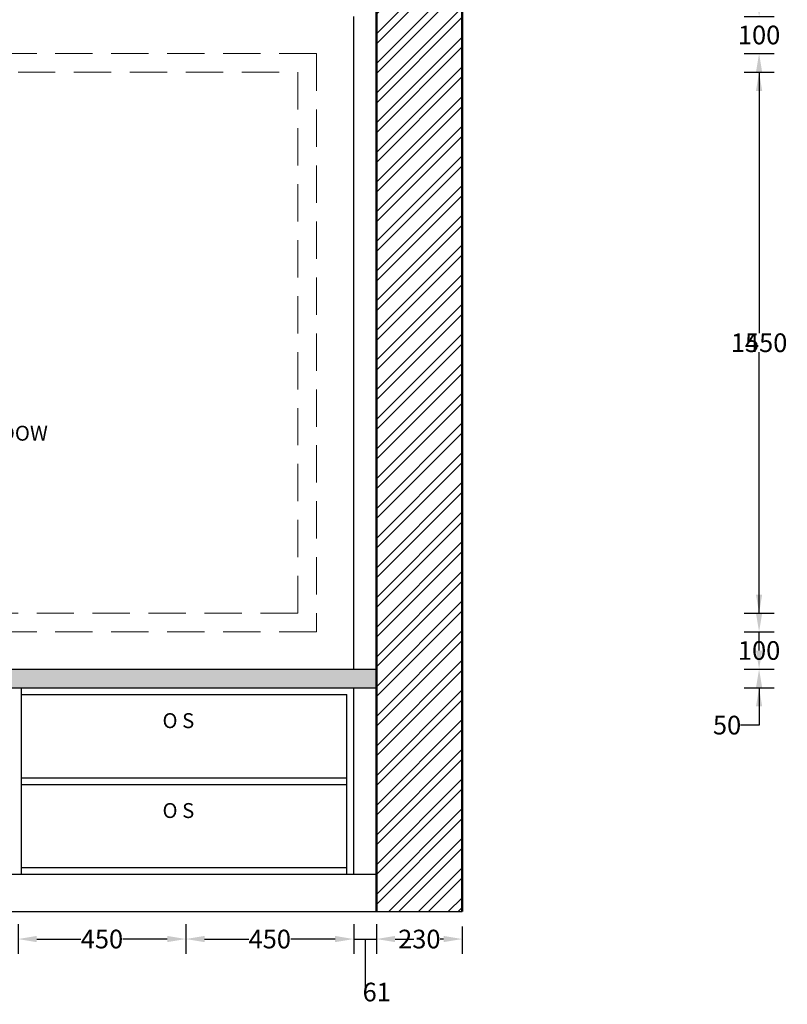
# Model space of a CAD drawing. Units: millimetres. Extents: x -472 to 16192, y -4730 to 4331.
# Tile 7 of 8: x 14134 to 16192, y -4534 to -1895. Entities that reach past the tile are written whole.
import ezdxf

# ---------------------------------------------------------------- set-up
doc = ezdxf.new("R2010")
doc.units = ezdxf.units.MM
doc.header["$MEASUREMENT"] = 0
doc.linetypes.add('DASHED', pattern=[0.75, 0.5, -0.25])
for name, color, linetype, lineweight in [('A-ANNO-DIMS', 2, 'Continuous', 18), ('A-ANNO-TEXT', 6, 'Continuous', 18), ('A-ELEV', 7, 'Continuous', 25), ('A-GLAZ', 4, 'DASHED', 18), ('A-WALL', 7, 'Continuous', 50), ('A-WALL-PATT', 8, 'Continuous', 13)]:
    doc.layers.add(name, color=color, linetype=linetype, lineweight=lineweight)
doc.styles.get("Standard").update_dxf_attribs({"font": 'arial.ttf'})
doc.dimstyles.get("Standard").update_dxf_attribs({"dimtxt": 50, "dimasz": 50, "dimexe": 40, "dimexo": 40, "dimgap": 0.09, "dimtad": 0, "dimtih": 1, "dimtoh": 1, "dimdec": 0, "dimzin": 0, "dimdsep": 46, "dimtxsty": 'Standard', "dimcen": 0.09, "dimclrd": 1, "dimclre": 3, "dimclrt": 6, "dimadec": 0, "dimazin": 0, "dimtfac": 1, "dimtdec": 0, "dimtofl": 0, "dimtmove": 0, "dimatfit": 3, "dimfxl": 40, "dimfxlon": 1, "dimtolj": 1, "dimtzin": 0, "dimarcsym": 0})

# ---------------------------------------------------------------- blocks, each defined once
blk = doc.blocks.new('*D61')
at = {"layer": 'A-ANNO-DIMS', "color": 0, "lineweight": -2, "transparency": 16777216}
for p, q in [((14129.7, -4319.4), (14129.7, -4399.4)), ((14579.7, -4319.4), (14579.7, -4399.4)), ((14179.7, -4359.4), (14298.4, -4359.4)), ((14529.7, -4359.4), (14410.9, -4359.4))]:
    blk.add_line(p, q, dxfattribs=at)
at = {"layer": 'A-ANNO-DIMS', "color": 0, "transparency": 16777216}
for points in [[(14179.7, -4351), (14179.7, -4367.7), (14129.7, -4359.4)], [(14529.7, -4351), (14529.7, -4367.7), (14579.7, -4359.4)]]:
    blk.add_solid(points, dxfattribs=at)
at = {"layer": 'Defpoints', "color": 0, "transparency": 16777216}
for p in [(14129.7, -4185.9), (14579.7, -4185.9), (14579.7, -4359.4)]:
    blk.add_point(p, dxfattribs=at)
at = {"layer": 'A-ANNO-DIMS', "color": 0, "transparency": 16777216, "insert": (14354.7, -4359.4), "char_height": 50, "attachment_point": 5}
blk.add_mtext('\\A1;450', dxfattribs=at)
blk = doc.blocks.new('*D62')
at = {"layer": 'A-ANNO-DIMS', "color": 0, "lineweight": -2, "transparency": 16777216}
for p, q in [((14579.7, -4319.4), (14579.7, -4399.4)), ((15029.7, -4319.4), (15029.7, -4399.4)), ((14629.7, -4359.4), (14748.4, -4359.4)), ((14979.7, -4359.4), (14860.9, -4359.4))]:
    blk.add_line(p, q, dxfattribs=at)
at = {"layer": 'A-ANNO-DIMS', "color": 0, "transparency": 16777216}
for points in [[(14629.7, -4351), (14629.7, -4367.7), (14579.7, -4359.4)], [(14979.7, -4351), (14979.7, -4367.7), (15029.7, -4359.4)]]:
    blk.add_solid(points, dxfattribs=at)
at = {"layer": 'Defpoints', "color": 0, "transparency": 16777216}
for p in [(14579.7, -4185.9), (15029.7, -4185.9), (15029.7, -4359.4)]:
    blk.add_point(p, dxfattribs=at)
at = {"layer": 'A-ANNO-DIMS', "color": 0, "transparency": 16777216, "insert": (14804.7, -4359.4), "char_height": 50, "attachment_point": 5}
blk.add_mtext('\\A1;450', dxfattribs=at)
blk = doc.blocks.new('*D63')
at = {"layer": 'A-ANNO-DIMS', "color": 0, "lineweight": -2, "transparency": 16777216}
for p, q in [((15029.7, -4319.4), (15029.7, -4399.4)), ((15090.7, -4319.4), (15090.7, -4399.4)), ((14979.7, -4359.4), (14929.7, -4359.4)), ((15029.7, -4359.4), (15090.7, -4359.4)), ((15060.2, -4359.4), (15060.2, -4501.5)), ((15140.7, -4359.4), (15190.7, -4359.4)), ((15060.2, -4501.5), (15060.3, -4501.5))]:
    blk.add_line(p, q, dxfattribs=at)
at = {"layer": 'A-ANNO-DIMS', "color": 0, "transparency": 16777216}
for points in [[(14979.7, -4351), (14979.7, -4367.7), (15029.7, -4359.4)], [(15140.7, -4351), (15140.7, -4367.7), (15090.7, -4359.4)]]:
    blk.add_solid(points, dxfattribs=at)
at = {"layer": 'Defpoints', "color": 0, "transparency": 16777216}
for p in [(15029.7, -4185.9), (15090.7, -4185.9), (15090.7, -4359.4)]:
    blk.add_point(p, dxfattribs=at)
at = {"layer": 'A-ANNO-DIMS', "color": 0, "transparency": 16777216, "insert": (15091.5, -4501.5), "char_height": 50, "attachment_point": 5}
blk.add_mtext('\\A1;61', dxfattribs=at)
blk = doc.blocks.new('*D64')
at = {"layer": 'A-ANNO-DIMS', "color": 0, "lineweight": -2, "transparency": 16777216}
for p, q in [((15090.7, -4319.4), (15090.7, -4399.4)), ((15320.7, -4325.9), (15320.7, -4399.4)), ((15140.7, -4359.4), (15150, -4359.4)), ((15270.7, -4359.4), (15261.3, -4359.4))]:
    blk.add_line(p, q, dxfattribs=at)
at = {"layer": 'A-ANNO-DIMS', "color": 0, "transparency": 16777216}
for points in [[(15140.7, -4351), (15140.7, -4367.7), (15090.7, -4359.4)], [(15270.7, -4351), (15270.7, -4367.7), (15320.7, -4359.4)]]:
    blk.add_solid(points, dxfattribs=at)
at = {"layer": 'Defpoints', "color": 0, "transparency": 16777216}
for p in [(15090.7, -4185.9), (15320.7, -4285.9), (15320.7, -4359.4)]:
    blk.add_point(p, dxfattribs=at)
at = {"layer": 'A-ANNO-DIMS', "color": 0, "transparency": 16777216, "insert": (15205.7, -4359.4), "char_height": 50, "attachment_point": 5}
blk.add_mtext('\\A1;230', dxfattribs=at)
blk = doc.blocks.new('*D100')
at = {"layer": 'A-ANNO-DIMS', "color": 1, "lineweight": -2, "transparency": 16777216}
for p, q in [((16116.7, -1835.9), (16116.7, -1785.9)), ((16116.7, -2035.9), (16116.7, -2085.9))]:
    blk.add_line(p, q, dxfattribs=at)
at = {"layer": 'A-ANNO-DIMS', "color": 3, "lineweight": -2, "transparency": 16777216}
for p, q in [((16076.7, -1885.9), (16156.7, -1885.9)), ((16076.7, -1985.9), (16156.7, -1985.9))]:
    blk.add_line(p, q, dxfattribs=at)
at = {"layer": 'A-ANNO-DIMS', "color": 1, "transparency": 16777216}
for points in [[(16108.3, -1835.9), (16125, -1835.9), (16116.7, -1885.9)], [(16108.3, -2035.9), (16125, -2035.9), (16116.7, -1985.9)]]:
    blk.add_solid(points, dxfattribs=at)
at = {"layer": 'Defpoints', "color": 0, "transparency": 16777216}
for p in [(5309, -1885.9), (5209, -1985.9), (16116.7, -1985.9)]:
    blk.add_point(p, dxfattribs=at)
at = {"layer": 'A-ANNO-DIMS', "color": 6, "transparency": 16777216, "insert": (16116.7, -1935.9), "char_height": 50, "attachment_point": 5}
blk.add_mtext('\\A1;100', dxfattribs=at)
blk = doc.blocks.new('*D101')
at = {"layer": 'A-ANNO-DIMS', "color": 3, "lineweight": -2, "transparency": 16777216}
for p, q in [((16076.7, -1985.9), (16156.7, -1985.9)), ((16076.7, -3535.9), (16156.7, -3535.9))]:
    blk.add_line(p, q, dxfattribs=at)
at = {"layer": 'A-ANNO-DIMS', "color": 1, "lineweight": -2, "transparency": 16777216}
for p, q in [((16116.7, -2035.9), (16116.7, -2735.3)), ((16116.7, -3485.9), (16116.7, -2786.5))]:
    blk.add_line(p, q, dxfattribs=at)
at = {"layer": 'A-ANNO-DIMS', "color": 1, "transparency": 16777216}
for points in [[(16108.3, -2035.9), (16125, -2035.9), (16116.7, -1985.9)], [(16108.3, -3485.9), (16125, -3485.9), (16116.7, -3535.9)]]:
    blk.add_solid(points, dxfattribs=at)
at = {"layer": 'Defpoints', "color": 0, "transparency": 16777216}
for p in [(5209, -1985.9), (5209, -3535.9), (16116.7, -3535.9)]:
    blk.add_point(p, dxfattribs=at)
at = {"layer": 'A-ANNO-DIMS', "color": 6, "transparency": 16777216, "insert": (16116.7, -2760.9), "char_height": 50, "attachment_point": 5}
blk.add_mtext('\\A1;1550', dxfattribs=at)
blk = doc.blocks.new('*D102')
at = {"layer": 'A-ANNO-DIMS', "color": 3, "lineweight": -2, "transparency": 16777216}
for p, q in [((16076.7, -2035.9), (16156.7, -2035.9)), ((16076.7, -3485.9), (16156.7, -3485.9))]:
    blk.add_line(p, q, dxfattribs=at)
at = {"layer": 'A-ANNO-DIMS', "color": 1, "lineweight": -2, "transparency": 16777216}
for p, q in [((16116.7, -2085.9), (16116.7, -2735.3)), ((16116.7, -3435.9), (16116.7, -2786.5))]:
    blk.add_line(p, q, dxfattribs=at)
at = {"layer": 'A-ANNO-DIMS', "color": 1, "transparency": 16777216}
for points in [[(16108.3, -2085.9), (16125, -2085.9), (16116.7, -2035.9)], [(16108.3, -3435.9), (16125, -3435.9), (16116.7, -3485.9)]]:
    blk.add_solid(points, dxfattribs=at)
at = {"layer": 'Defpoints', "color": 0, "transparency": 16777216}
for p in [(5159, -2035.9), (5159, -3485.9), (16116.7, -3485.9)]:
    blk.add_point(p, dxfattribs=at)
at = {"layer": 'A-ANNO-DIMS', "color": 6, "transparency": 16777216, "insert": (16116.7, -2760.9), "char_height": 50, "attachment_point": 5}
blk.add_mtext('\\A1;1450', dxfattribs=at)
blk = doc.blocks.new('*D103')
at = {"layer": 'A-ANNO-DIMS', "color": 1, "lineweight": -2, "transparency": 16777216}
for p, q in [((16116.7, -3485.9), (16116.7, -3435.9)), ((16116.7, -3685.9), (16116.7, -3735.9))]:
    blk.add_line(p, q, dxfattribs=at)
at = {"layer": 'A-ANNO-DIMS', "color": 3, "lineweight": -2, "transparency": 16777216}
for p, q in [((16076.7, -3535.9), (16156.7, -3535.9)), ((16076.7, -3635.9), (16156.7, -3635.9))]:
    blk.add_line(p, q, dxfattribs=at)
at = {"layer": 'A-ANNO-DIMS', "color": 1, "transparency": 16777216}
for points in [[(16108.3, -3485.9), (16125, -3485.9), (16116.7, -3535.9)], [(16108.3, -3685.9), (16125, -3685.9), (16116.7, -3635.9)]]:
    blk.add_solid(points, dxfattribs=at)
at = {"layer": 'Defpoints', "color": 0, "transparency": 16777216}
for p in [(5209, -3535.9), (5309, -3635.9), (16116.7, -3635.9)]:
    blk.add_point(p, dxfattribs=at)
at = {"layer": 'A-ANNO-DIMS', "color": 6, "transparency": 16777216, "insert": (16116.7, -3585.9), "char_height": 50, "attachment_point": 5}
blk.add_mtext('\\A1;100', dxfattribs=at)
blk = doc.blocks.new('*D104')
at = {"layer": 'A-ANNO-DIMS', "color": 1, "lineweight": -2, "transparency": 16777216}
for p, q in [((16116.7, -3585.9), (16116.7, -3535.9)), ((16116.7, -3735.9), (16116.7, -3785.9)), ((16116.7, -3785.9), (16066.7, -3785.9))]:
    blk.add_line(p, q, dxfattribs=at)
at = {"layer": 'A-ANNO-DIMS', "color": 3, "lineweight": -2, "transparency": 16777216}
for p, q in [((16076.7, -3635.9), (16156.7, -3635.9)), ((16076.7, -3685.9), (16156.7, -3685.9))]:
    blk.add_line(p, q, dxfattribs=at)
at = {"layer": 'A-ANNO-DIMS', "color": 1, "transparency": 16777216}
for points in [[(16108.3, -3585.9), (16125, -3585.9), (16116.7, -3635.9)], [(16108.3, -3735.9), (16125, -3735.9), (16116.7, -3685.9)]]:
    blk.add_solid(points, dxfattribs=at)
at = {"layer": 'Defpoints', "color": 0, "transparency": 16777216}
for p in [(5309, -3635.9), (5309, -3685.9), (16116.7, -3685.9)]:
    blk.add_point(p, dxfattribs=at)
at = {"layer": 'A-ANNO-DIMS', "color": 6, "transparency": 16777216, "insert": (16030.8, -3785.9), "char_height": 50, "attachment_point": 5}
blk.add_mtext('\\A1;50', dxfattribs=at)
blk = doc.blocks.new('*D105')
at = {"layer": 'A-ANNO-DIMS', "color": 3, "lineweight": -2, "transparency": 16777216}
for p, q in [((14929.7, -534.9), (14929.7, -454.9)), ((15029.7, -534.9), (15029.7, -454.9))]:
    blk.add_line(p, q, dxfattribs=at)
at = {"layer": 'A-ANNO-DIMS', "color": 1, "lineweight": -2, "transparency": 16777216}
for p, q in [((14879.7, -494.9), (14829.7, -494.9)), ((15079.7, -494.9), (15129.7, -494.9))]:
    blk.add_line(p, q, dxfattribs=at)
at = {"layer": 'A-ANNO-DIMS', "color": 1, "transparency": 16777216}
for points in [[(14879.7, -486.6), (14879.7, -503.2), (14929.7, -494.9)], [(15079.7, -486.6), (15079.7, -503.2), (15029.7, -494.9)]]:
    blk.add_solid(points, dxfattribs=at)
at = {"layer": 'Defpoints', "color": 0, "transparency": 16777216}
for p in [(15029.7, -494.9), (15029.7, -1885.9), (14929.7, -1985.9)]:
    blk.add_point(p, dxfattribs=at)
at = {"layer": 'A-ANNO-DIMS', "color": 6, "transparency": 16777216, "insert": (15182.5, -494.9), "char_height": 50, "attachment_point": 5}
blk.add_mtext('\\A1;100', dxfattribs=at)
blk = doc.blocks.new('*D106')
at = {"layer": 'A-ANNO-DIMS', "color": 3, "lineweight": -2, "transparency": 16777216}
for p, q in [((13329.7, -534.9), (13329.7, -454.9)), ((14929.7, -534.9), (14929.7, -454.9))]:
    blk.add_line(p, q, dxfattribs=at)
at = {"layer": 'A-ANNO-DIMS', "color": 1, "lineweight": -2, "transparency": 16777216}
for p, q in [((13379.7, -494.9), (14057.3, -494.9)), ((14879.7, -494.9), (14202, -494.9))]:
    blk.add_line(p, q, dxfattribs=at)
at = {"layer": 'A-ANNO-DIMS', "color": 1, "transparency": 16777216}
for points in [[(13379.7, -486.6), (13379.7, -503.2), (13329.7, -494.9)], [(14879.7, -486.6), (14879.7, -503.2), (14929.7, -494.9)]]:
    blk.add_solid(points, dxfattribs=at)
at = {"layer": 'Defpoints', "color": 0, "transparency": 16777216}
for p in [(14929.7, -494.9), (13329.7, -1985.9), (14929.7, -1985.9)]:
    blk.add_point(p, dxfattribs=at)
at = {"layer": 'A-ANNO-DIMS', "color": 6, "transparency": 16777216, "insert": (14129.7, -494.9), "char_height": 50, "attachment_point": 5}
blk.add_mtext('\\A1;1600', dxfattribs=at)
blk = doc.blocks.new('*D107')
at = {"layer": 'A-ANNO-DIMS', "color": 3, "lineweight": -2, "transparency": 16777216}
for p, q in [((13379.7, -534.9), (13379.7, -454.9)), ((14879.7, -534.9), (14879.7, -454.9))]:
    blk.add_line(p, q, dxfattribs=at)
at = {"layer": 'A-ANNO-DIMS', "color": 1, "lineweight": -2, "transparency": 16777216}
for p, q in [((13429.7, -494.9), (14057.3, -494.9)), ((14829.7, -494.9), (14202, -494.9))]:
    blk.add_line(p, q, dxfattribs=at)
at = {"layer": 'A-ANNO-DIMS', "color": 1, "transparency": 16777216}
for points in [[(13429.7, -486.6), (13429.7, -503.2), (13379.7, -494.9)], [(14829.7, -486.6), (14829.7, -503.2), (14879.7, -494.9)]]:
    blk.add_solid(points, dxfattribs=at)
at = {"layer": 'Defpoints', "color": 0, "transparency": 16777216}
for p in [(14879.7, -494.9), (13379.7, -2035.9), (14879.7, -2035.9)]:
    blk.add_point(p, dxfattribs=at)
at = {"layer": 'A-ANNO-DIMS', "color": 6, "transparency": 16777216, "insert": (14129.7, -494.9), "char_height": 50, "attachment_point": 5}
blk.add_mtext('\\A1;1500', dxfattribs=at)
blk = doc.blocks.new('*D108')
at = {"layer": 'A-ANNO-DIMS', "color": 1, "lineweight": -2, "transparency": 16777216}
for p, q in [((16116.7, -1835.9), (16116.7, -1785.9)), ((16116.7, -2035.9), (16116.7, -2085.9))]:
    blk.add_line(p, q, dxfattribs=at)
at = {"layer": 'A-ANNO-DIMS', "color": 3, "lineweight": -2, "transparency": 16777216}
for p, q in [((16076.7, -1885.9), (16156.7, -1885.9)), ((16076.7, -1985.9), (16156.7, -1985.9))]:
    blk.add_line(p, q, dxfattribs=at)
at = {"layer": 'A-ANNO-DIMS', "color": 1, "transparency": 16777216}
for points in [[(16108.3, -1835.9), (16125, -1835.9), (16116.7, -1885.9)], [(16108.3, -2035.9), (16125, -2035.9), (16116.7, -1985.9)]]:
    blk.add_solid(points, dxfattribs=at)
at = {"layer": 'Defpoints', "color": 0, "transparency": 16777216}
for p in [(15029.7, -1885.9), (14929.7, -1985.9), (16116.7, -1985.9)]:
    blk.add_point(p, dxfattribs=at)
at = {"layer": 'A-ANNO-DIMS', "color": 6, "transparency": 16777216, "insert": (16116.7, -1935.9), "char_height": 50, "attachment_point": 5}
blk.add_mtext('\\A1;100', dxfattribs=at)
blk = doc.blocks.new('*D109')
at = {"layer": 'A-ANNO-DIMS', "color": 3, "lineweight": -2, "transparency": 16777216}
for p, q in [((16076.7, -1985.9), (16156.7, -1985.9)), ((16076.7, -3535.9), (16156.7, -3535.9))]:
    blk.add_line(p, q, dxfattribs=at)
at = {"layer": 'A-ANNO-DIMS', "color": 1, "lineweight": -2, "transparency": 16777216}
for p, q in [((16116.7, -2035.9), (16116.7, -2735.3)), ((16116.7, -3485.9), (16116.7, -2786.5))]:
    blk.add_line(p, q, dxfattribs=at)
at = {"layer": 'A-ANNO-DIMS', "color": 1, "transparency": 16777216}
for points in [[(16108.3, -2035.9), (16125, -2035.9), (16116.7, -1985.9)], [(16108.3, -3485.9), (16125, -3485.9), (16116.7, -3535.9)]]:
    blk.add_solid(points, dxfattribs=at)
at = {"layer": 'Defpoints', "color": 0, "transparency": 16777216}
for p in [(14929.7, -1985.9), (14929.7, -3535.9), (16116.7, -3535.9)]:
    blk.add_point(p, dxfattribs=at)
at = {"layer": 'A-ANNO-DIMS', "color": 6, "transparency": 16777216, "insert": (16116.7, -2760.9), "char_height": 50, "attachment_point": 5}
blk.add_mtext('\\A1;1550', dxfattribs=at)
blk = doc.blocks.new('*D110')
at = {"layer": 'A-ANNO-DIMS', "color": 3, "lineweight": -2, "transparency": 16777216}
for p, q in [((16076.7, -2035.9), (16156.7, -2035.9)), ((16076.7, -3485.9), (16156.7, -3485.9))]:
    blk.add_line(p, q, dxfattribs=at)
at = {"layer": 'A-ANNO-DIMS', "color": 1, "lineweight": -2, "transparency": 16777216}
for p, q in [((16116.7, -2085.9), (16116.7, -2735.3)), ((16116.7, -3435.9), (16116.7, -2786.5))]:
    blk.add_line(p, q, dxfattribs=at)
at = {"layer": 'A-ANNO-DIMS', "color": 1, "transparency": 16777216}
for points in [[(16108.3, -2085.9), (16125, -2085.9), (16116.7, -2035.9)], [(16108.3, -3435.9), (16125, -3435.9), (16116.7, -3485.9)]]:
    blk.add_solid(points, dxfattribs=at)
at = {"layer": 'Defpoints', "color": 0, "transparency": 16777216}
for p in [(14879.7, -2035.9), (14879.7, -3485.9), (16116.7, -3485.9)]:
    blk.add_point(p, dxfattribs=at)
at = {"layer": 'A-ANNO-DIMS', "color": 6, "transparency": 16777216, "insert": (16116.7, -2760.9), "char_height": 50, "attachment_point": 5}
blk.add_mtext('\\A1;1450', dxfattribs=at)
blk = doc.blocks.new('*D111')
at = {"layer": 'A-ANNO-DIMS', "color": 1, "lineweight": -2, "transparency": 16777216}
for p, q in [((16116.7, -3485.9), (16116.7, -3435.9)), ((16116.7, -3685.9), (16116.7, -3735.9))]:
    blk.add_line(p, q, dxfattribs=at)
at = {"layer": 'A-ANNO-DIMS', "color": 3, "lineweight": -2, "transparency": 16777216}
for p, q in [((16076.7, -3535.9), (16156.7, -3535.9)), ((16076.7, -3635.9), (16156.7, -3635.9))]:
    blk.add_line(p, q, dxfattribs=at)
at = {"layer": 'A-ANNO-DIMS', "color": 1, "transparency": 16777216}
for points in [[(16108.3, -3485.9), (16125, -3485.9), (16116.7, -3535.9)], [(16108.3, -3685.9), (16125, -3685.9), (16116.7, -3635.9)]]:
    blk.add_solid(points, dxfattribs=at)
at = {"layer": 'Defpoints', "color": 0, "transparency": 16777216}
for p in [(14929.7, -3535.9), (15029.7, -3635.9), (16116.7, -3635.9)]:
    blk.add_point(p, dxfattribs=at)
at = {"layer": 'A-ANNO-DIMS', "color": 6, "transparency": 16777216, "insert": (16116.7, -3585.9), "char_height": 50, "attachment_point": 5}
blk.add_mtext('\\A1;100', dxfattribs=at)
blk = doc.blocks.new('*D112')
at = {"layer": 'A-ANNO-DIMS', "color": 1, "lineweight": -2, "transparency": 16777216}
for p, q in [((16116.7, -3585.9), (16116.7, -3535.9)), ((16116.7, -3735.9), (16116.7, -3785.9)), ((16116.7, -3785.9), (16066.7, -3785.9))]:
    blk.add_line(p, q, dxfattribs=at)
at = {"layer": 'A-ANNO-DIMS', "color": 3, "lineweight": -2, "transparency": 16777216}
for p, q in [((16076.7, -3635.9), (16156.7, -3635.9)), ((16076.7, -3685.9), (16156.7, -3685.9))]:
    blk.add_line(p, q, dxfattribs=at)
at = {"layer": 'A-ANNO-DIMS', "color": 1, "transparency": 16777216}
for points in [[(16108.3, -3585.9), (16125, -3585.9), (16116.7, -3635.9)], [(16108.3, -3735.9), (16125, -3735.9), (16116.7, -3685.9)]]:
    blk.add_solid(points, dxfattribs=at)
at = {"layer": 'Defpoints', "color": 0, "transparency": 16777216}
for p in [(15029.7, -3635.9), (15029.7, -3685.9), (16116.7, -3685.9)]:
    blk.add_point(p, dxfattribs=at)
at = {"layer": 'A-ANNO-DIMS', "color": 6, "transparency": 16777216, "insert": (16030.8, -3785.9), "char_height": 50, "attachment_point": 5}
blk.add_mtext('\\A1;50', dxfattribs=at)

msp = doc.modelspace()

# ---------------------------------------------------------------- hatches: boundary and pattern name
at = {"layer": 'A-GLAZ'}
h = msp.add_hatch(color=256, dxfattribs=at)
h.dxf.hatch_style = 1
h.paths.add_polyline_path([(15090.7, -3635.9), (13229.7, -3635.9), (13229.7, -3685.9), (15029.7, -3685.9), (15090.7, -3685.9)])
at = {"layer": 'A-WALL-PATT'}
h = msp.add_hatch(dxfattribs=at)
h.set_pattern_fill('ANSI32', color=256, scale=150)
h.paths.add_polyline_path([(9720.7, -1290.9), (9720.7, -4285.9), (9950.7, -4285.9), (9950.7, -4185.9), (9950.7, -1885.9), (9950.7, -1290.9)])
h.paths.add_polyline_path([(5370, -4285.9), (5600, -4285.9), (5600, -1290.9), (5370, -1290.9)])
h.paths.add_polyline_path([(15320.7, -1290.9), (15090.7, -1290.9), (15090.7, -4285.9), (15320.7, -4285.9)])
h.paths.add_polyline_path([(0, -4285.9), (230, -4285.9), (230, -4185.9), (230, -1885.9), (230, -1290.9), (0, -1290.9)])

# ---------------------------------------------------------------- linework, layer by layer
at = {"layer": 'A-ELEV'}
for p, q in [((15029.7, -3635.9), (15029.7, -1885.9)), ((13229.7, -3635.9), (15090.7, -3635.9)), ((13229.7, -3685.9), (15090.7, -3685.9)), ((14138.7, -4185.9), (14138.7, -3685.9)), ((15029.7, -4185.9), (15029.7, -3685.9)), ((14138.7, -3703.9), (15011.7, -3703.9)), ((15011.7, -4185.9), (15011.7, -3703.9)), ((14138.7, -3926.9), (15011.7, -3926.9)), ((14138.7, -3944.9), (15011.7, -3944.9)), ((14138.7, -4167.9), (15011.7, -4167.9)), ((13229.7, -4185.9), (15090.7, -4185.9)), ((9720.7, -4285.9), (15320.7, -4285.9))]:
    msp.add_line(p, q, dxfattribs=at)
at = {"layer": 'A-GLAZ', "ltscale": 200}
for points in [[(13329.7, -1985.9), (14929.7, -1985.9), (14929.7, -3535.9), (13329.7, -3535.9)], [(13379.7, -2035.9), (14879.7, -2035.9), (14879.7, -3485.9), (13379.7, -3485.9)]]:
    msp.add_lwpolyline(points, close=True, dxfattribs=at)
at = {"layer": 'A-WALL'}
for p, q in [((15090.7, -4285.9), (15090.7, -1290.9)), ((15320.7, -4285.9), (15320.7, -1290.9))]:
    msp.add_line(p, q, dxfattribs=at)

# ---------------------------------------------------------------- texts
at = {"layer": 'A-ANNO-TEXT', "char_height": 40, "attachment_point": 1}
for s, insert in [('WINDOW', (13980.3, -2983.4)), ('O S', (14517, -3753.9)), ('O S', (14517, -3994.9))]:
    msp.add_mtext_dynamic_manual_height_columns(s, width=327.678, gutter_width=1, heights=[0], dxfattribs=dict(at, insert=insert))

# ---------------------------------------------------------------- dimensions: what is measured, and where the dimension line sits
at = {"layer": 'A-ANNO-DIMS'}
for base, p1, p2, override, picture, middle in [((14929.7, -494.9), (13329.7, -1985.9), (14929.7, -1985.9), {"dimdec": 0, "dimlfac": 1, "dimrnd": 0, "dimzin": 0, "dimdsep": 46, "dimlunit": 2}, '*D106', (14129.7, -494.9)), ((14879.7, -494.9), (13379.7, -2035.9), (14879.7, -2035.9), {"dimdec": 0, "dimlfac": 1, "dimrnd": 0, "dimzin": 0, "dimdsep": 46, "dimlunit": 2}, '*D107', (14129.7, -494.9)), ((15029.7, -494.9), (14929.7, -1985.9), (15029.7, -1885.9), {"dimdec": 0, "dimlfac": 1, "dimrnd": 0, "dimzin": 0, "dimdsep": 46, "dimlunit": 2}, '*D105', (15182.5, -494.9)), ((14579.7, -4359.4), (14129.7, -4185.9), (14579.7, -4185.9), {"dimclrd": 0, "dimclre": 0, "dimclrt": 0, "dimtmove": 1}, '*D61', (14354.7, -4359.4)), ((15029.7, -4359.4), (14579.7, -4185.9), (15029.7, -4185.9), {"dimclrd": 0, "dimclre": 0, "dimclrt": 0, "dimtmove": 1}, '*D62', (14804.7, -4359.4)), ((15090.7, -4359.4), (15029.7, -4185.9), (15090.7, -4185.9), {"dimclrd": 0, "dimclre": 0, "dimclrt": 0, "dimtmove": 1}, '*D63', (15060.4, -4501.5)), ((15320.7, -4359.4), (15090.7, -4185.9), (15320.7, -4285.9), {"dimclrd": 0, "dimclre": 0, "dimclrt": 0, "dimtmove": 1}, '*D64', (15205.7, -4359.4))]:
    dim = msp.add_linear_dim(base=base, p1=p1, p2=p2, dimstyle='Standard', override=override, dxfattribs=at)
    dim.commit()
    dim.dimension.update_dxf_attribs({"geometry": picture, "text_midpoint": middle})
for base, p1, p2, picture, middle in [((16116.7, -1985.9), (5309, -1885.9), (5209, -1985.9), '*D100', (16116.7, -1935.9)), ((16116.7, -1985.9), (15029.7, -1885.9), (14929.7, -1985.9), '*D108', (16116.7, -1935.9)), ((16116.7, -3535.9), (5209, -1985.9), (5209, -3535.9), '*D101', (16116.7, -2760.9)), ((16116.7, -3535.9), (14929.7, -1985.9), (14929.7, -3535.9), '*D109', (16116.7, -2760.9)), ((16116.7, -3485.9), (5159, -2035.9), (5159, -3485.9), '*D102', (16116.7, -2760.9)), ((16116.7, -3485.9), (14879.7, -2035.9), (14879.7, -3485.9), '*D110', (16116.7, -2760.9)), ((16116.7, -3635.9), (5209, -3535.9), (5309, -3635.9), '*D103', (16116.7, -3585.9)), ((16116.7, -3635.9), (14929.7, -3535.9), (15029.7, -3635.9), '*D111', (16116.7, -3585.9)), ((16116.7, -3685.9), (5309, -3635.9), (5309, -3685.9), '*D104', (16030.8, -3785.9)), ((16116.7, -3685.9), (15029.7, -3635.9), (15029.7, -3685.9), '*D112', (16030.8, -3785.9))]:
    dim = msp.add_linear_dim(base=base, p1=p1, p2=p2, angle=90, dimstyle='Standard', override={"dimdec": 0, "dimlfac": 1, "dimrnd": 0, "dimzin": 0, "dimdsep": 46, "dimlunit": 2}, dxfattribs=at)
    dim.commit()
    dim.dimension.update_dxf_attribs({"geometry": picture, "text_midpoint": middle})

doc.saveas('drawing.dxf')
